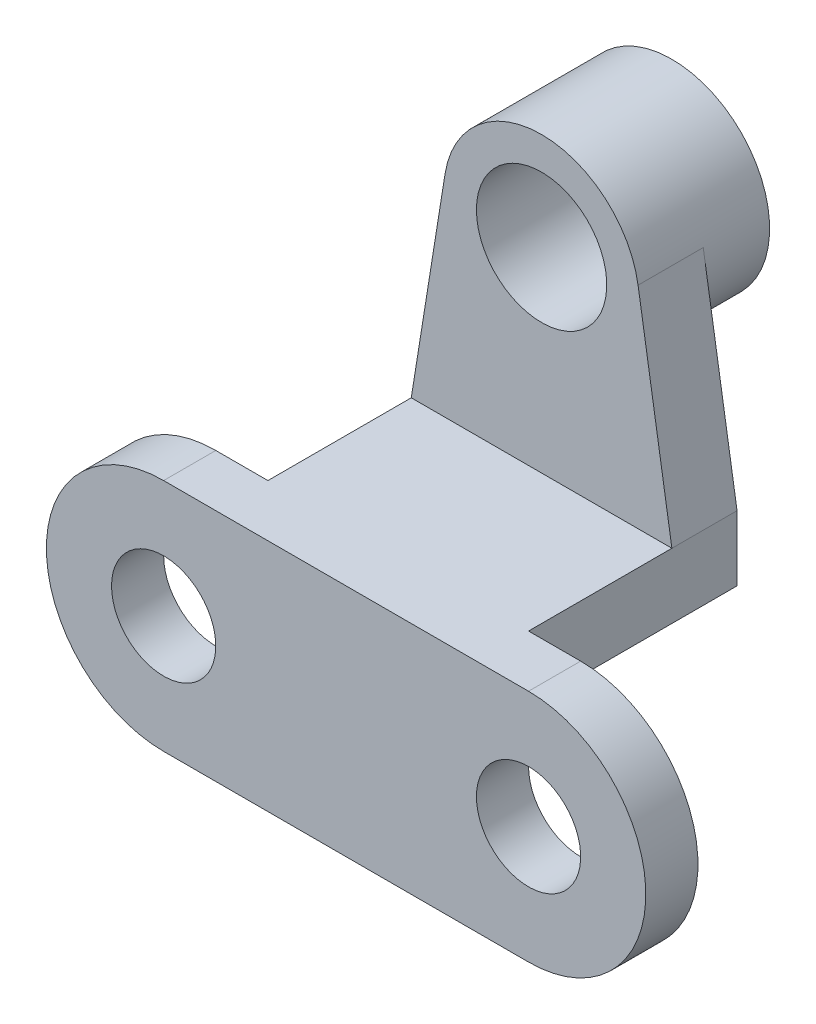
ISO-10303-21;
HEADER;
FILE_DESCRIPTION(('STEP AP214'),'2;1');
FILE_NAME('part.step','',(''),(''),'','','');
FILE_SCHEMA(('AUTOMOTIVE_DESIGN { 1 0 10303 214 1 1 1 1 }'));
ENDSEC;
DATA;
#1=APPLICATION_CONTEXT('core data for automotive mechanical design processes');
#2=APPLICATION_PROTOCOL_DEFINITION('international standard','automotive_design',2000,#1);
#3=PRODUCT_CONTEXT('',#1,'mechanical');
#4=PRODUCT('Part','Part','',(#3));
#5=PRODUCT_RELATED_PRODUCT_CATEGORY('part','',(#4));
#6=PRODUCT_DEFINITION_FORMATION('','',#4);
#7=PRODUCT_DEFINITION_CONTEXT('part definition',#1,'design');
#8=PRODUCT_DEFINITION('design','',#6,#7);
#9=PRODUCT_DEFINITION_SHAPE('','',#8);
#10=(LENGTH_UNIT() NAMED_UNIT(*) SI_UNIT(.MILLI.,.METRE.));
#11=(NAMED_UNIT(*) PLANE_ANGLE_UNIT() SI_UNIT($,.RADIAN.));
#12=(NAMED_UNIT(*) SI_UNIT($,.STERADIAN.) SOLID_ANGLE_UNIT());
#13=UNCERTAINTY_MEASURE_WITH_UNIT(LENGTH_MEASURE(1.E-05),#10,'distance_accuracy_value','');
#14=(GEOMETRIC_REPRESENTATION_CONTEXT(3) GLOBAL_UNCERTAINTY_ASSIGNED_CONTEXT((#13)) GLOBAL_UNIT_ASSIGNED_CONTEXT((#10,
#11,#12)) REPRESENTATION_CONTEXT('',''));
#15=CARTESIAN_POINT('',(0.,0.,0.));
#16=DIRECTION('',(0.,0.,1.));
#17=DIRECTION('',(1.,0.,0.));
#18=AXIS2_PLACEMENT_3D('',#15,#16,#17);
#19=CARTESIAN_POINT('',(66.,0.,0.));
#20=DIRECTION('',(0.,-0.776114000116266,-0.630592625094466));
#21=DIRECTION('',(0.,0.630592625094466,-0.776114000116266));
#22=AXIS2_PLACEMENT_3D('',#19,#20,#21);
#23=PLANE('',#22);
#24=DIRECTION('',(0.,0.630592625094466,-0.776114000116266));
#25=VECTOR('',#24,1.);
#26=CARTESIAN_POINT('',(52.,0.,0.));
#27=LINE('',#26,#25);
#28=CARTESIAN_POINT('',(52.,0.,0.));
#29=VERTEX_POINT('',#28);
#30=CARTESIAN_POINT('',(52.,26.,-32.));
#31=VERTEX_POINT('',#30);
#32=EDGE_CURVE('E199',#29,#31,#27,.T.);
#33=ORIENTED_EDGE('',*,*,#32,.F.);
#34=DIRECTION('',(-1.,0.,0.));
#35=VECTOR('',#34,1.);
#36=CARTESIAN_POINT('',(66.,0.,0.));
#37=LINE('',#36,#35);
#38=CARTESIAN_POINT('',(40.,0.,0.));
#39=VERTEX_POINT('',#38);
#40=EDGE_CURVE('E268',#29,#39,#37,.T.);
#41=ORIENTED_EDGE('',*,*,#40,.T.);
#42=DIRECTION('',(0.,-0.630592625094466,0.776114000116266));
#43=VECTOR('',#42,1.);
#44=CARTESIAN_POINT('',(40.,0.,0.));
#45=LINE('',#44,#43);
#46=CARTESIAN_POINT('',(40.,26.,-32.));
#47=VERTEX_POINT('',#46);
#48=EDGE_CURVE('E208',#47,#39,#45,.T.);
#49=ORIENTED_EDGE('',*,*,#48,.F.);
#50=DIRECTION('',(-1.,0.,0.));
#51=VECTOR('',#50,1.);
#52=CARTESIAN_POINT('',(26.,26.,-32.));
#53=LINE('',#52,#51);
#54=EDGE_CURVE('E99',#31,#47,#53,.T.);
#55=ORIENTED_EDGE('',*,*,#54,.F.);
#56=EDGE_LOOP('',(#33,#41,#49,#55));
#57=FACE_BOUND('',#56,.T.);
#58=ADVANCED_FACE('F84',(#57),#23,.T.);
#59=CARTESIAN_POINT('',(0.,0.,0.));
#60=DIRECTION('',(0.,0.,-1.));
#61=DIRECTION('',(-1.,0.,0.));
#62=AXIS2_PLACEMENT_3D('',#59,#60,#61);
#63=PLANE('',#62);
#64=DIRECTION('',(1.,0.,0.));
#65=VECTOR('',#64,1.);
#66=CARTESIAN_POINT('',(52.,26.,0.));
#67=LINE('',#66,#65);
#68=CARTESIAN_POINT('',(52.,26.,0.));
#69=VERTEX_POINT('',#68);
#70=CARTESIAN_POINT('',(66.,26.,0.));
#71=VERTEX_POINT('',#70);
#72=EDGE_CURVE('E193',#69,#71,#67,.T.);
#73=ORIENTED_EDGE('',*,*,#72,.T.);
#74=DIRECTION('',(0.,1.,0.));
#75=VECTOR('',#74,1.);
#76=CARTESIAN_POINT('',(66.,26.,0.));
#77=LINE('',#76,#75);
#78=CARTESIAN_POINT('',(66.,36.,0.));
#79=VERTEX_POINT('',#78);
#80=EDGE_CURVE('E220',#71,#79,#77,.T.);
#81=ORIENTED_EDGE('',*,*,#80,.T.);
#82=DIRECTION('',(-1.,0.,0.));
#83=VECTOR('',#82,1.);
#84=CARTESIAN_POINT('',(0.,36.,0.));
#85=LINE('',#84,#83);
#86=CARTESIAN_POINT('',(74.,36.,0.));
#87=VERTEX_POINT('',#86);
#88=EDGE_CURVE('E90',#87,#79,#85,.T.);
#89=ORIENTED_EDGE('',*,*,#88,.F.);
#90=CARTESIAN_POINT('',(74.,18.,0.));
#91=DIRECTION('',(0.,0.,1.));
#92=DIRECTION('',(1.,0.,0.));
#93=AXIS2_PLACEMENT_3D('',#90,#91,#92);
#94=CIRCLE('',#93,18.);
#95=CARTESIAN_POINT('',(74.,0.,0.));
#96=VERTEX_POINT('',#95);
#97=EDGE_CURVE('E249',#96,#87,#94,.T.);
#98=ORIENTED_EDGE('',*,*,#97,.F.);
#99=DIRECTION('',(1.,0.,0.));
#100=VECTOR('',#99,1.);
#101=CARTESIAN_POINT('',(0.,0.,0.));
#102=LINE('',#101,#100);
#103=EDGE_CURVE('E248',#29,#96,#102,.T.);
#104=ORIENTED_EDGE('',*,*,#103,.F.);
#105=DIRECTION('',(0.,-1.,0.));
#106=VECTOR('',#105,1.);
#107=CARTESIAN_POINT('',(52.,26.,0.));
#108=LINE('',#107,#106);
#109=EDGE_CURVE('E197',#69,#29,#108,.T.);
#110=ORIENTED_EDGE('',*,*,#109,.F.);
#111=EDGE_LOOP('',(#73,#81,#89,#98,#104,#110));
#112=FACE_BOUND('',#111,.T.);
#113=CARTESIAN_POINT('',(74.,18.,0.));
#114=DIRECTION('',(0.,0.,-1.));
#115=DIRECTION('',(-1.,0.,0.));
#116=AXIS2_PLACEMENT_3D('',#113,#114,#115);
#117=CIRCLE('',#116,8.);
#118=CARTESIAN_POINT('',(66.,18.,0.));
#119=VERTEX_POINT('',#118);
#120=EDGE_CURVE('E311',#119,#119,#117,.T.);
#121=ORIENTED_EDGE('',*,*,#120,.F.);
#122=EDGE_LOOP('',(#121));
#123=FACE_BOUND('',#122,.T.);
#124=ADVANCED_FACE('F275',(#112,#123),#63,.T.);
#125=CARTESIAN_POINT('',(0.,36.,8.));
#126=DIRECTION('',(0.,-1.,0.));
#127=DIRECTION('',(0.,0.,-1.));
#128=AXIS2_PLACEMENT_3D('',#125,#126,#127);
#129=PLANE('',#128);
#130=DIRECTION('',(1.,0.,0.));
#131=VECTOR('',#130,1.);
#132=CARTESIAN_POINT('',(0.,36.,-22.));
#133=LINE('',#132,#131);
#134=CARTESIAN_POINT('',(26.,36.,-22.));
#135=VERTEX_POINT('',#134);
#136=CARTESIAN_POINT('',(66.,36.,-22.));
#137=VERTEX_POINT('',#136);
#138=EDGE_CURVE('E108',#135,#137,#133,.T.);
#139=ORIENTED_EDGE('',*,*,#138,.F.);
#140=DIRECTION('',(0.,0.,1.));
#141=VECTOR('',#140,1.);
#142=CARTESIAN_POINT('',(26.,36.,0.));
#143=LINE('',#142,#141);
#144=CARTESIAN_POINT('',(26.,36.,0.));
#145=VERTEX_POINT('',#144);
#146=EDGE_CURVE('E225',#135,#145,#143,.T.);
#147=ORIENTED_EDGE('',*,*,#146,.T.);
#148=CARTESIAN_POINT('',(18.,36.,0.));
#149=VERTEX_POINT('',#148);
#150=EDGE_CURVE('E261',#145,#149,#85,.T.);
#151=ORIENTED_EDGE('',*,*,#150,.T.);
#152=DIRECTION('',(0.,0.,1.));
#153=VECTOR('',#152,1.);
#154=CARTESIAN_POINT('',(18.,36.,0.));
#155=LINE('',#154,#153);
#156=CARTESIAN_POINT('',(18.,36.,8.));
#157=VERTEX_POINT('',#156);
#158=EDGE_CURVE('E243',#149,#157,#155,.T.);
#159=ORIENTED_EDGE('',*,*,#158,.T.);
#160=DIRECTION('',(-1.,0.,0.));
#161=VECTOR('',#160,1.);
#162=CARTESIAN_POINT('',(0.,36.,8.));
#163=LINE('',#162,#161);
#164=CARTESIAN_POINT('',(74.,36.,8.));
#165=VERTEX_POINT('',#164);
#166=EDGE_CURVE('E92',#165,#157,#163,.T.);
#167=ORIENTED_EDGE('',*,*,#166,.F.);
#168=DIRECTION('',(0.,0.,1.));
#169=VECTOR('',#168,1.);
#170=CARTESIAN_POINT('',(74.,36.,0.));
#171=LINE('',#170,#169);
#172=EDGE_CURVE('E246',#87,#165,#171,.T.);
#173=ORIENTED_EDGE('',*,*,#172,.F.);
#174=ORIENTED_EDGE('',*,*,#88,.T.);
#175=DIRECTION('',(0.,0.,-1.));
#176=VECTOR('',#175,1.);
#177=CARTESIAN_POINT('',(66.,36.,-32.));
#178=LINE('',#177,#176);
#179=EDGE_CURVE('E224',#79,#137,#178,.T.);
#180=ORIENTED_EDGE('',*,*,#179,.T.);
#181=EDGE_LOOP('',(#139,#147,#151,#159,#167,#173,#174,#180));
#182=FACE_BOUND('',#181,.T.);
#183=ADVANCED_FACE('F281',(#182),#129,.F.);
#184=CARTESIAN_POINT('',(0.,0.,8.));
#185=DIRECTION('',(0.,0.,-1.));
#186=DIRECTION('',(-1.,0.,0.));
#187=AXIS2_PLACEMENT_3D('',#184,#185,#186);
#188=PLANE('',#187);
#189=CARTESIAN_POINT('',(74.,18.,8.));
#190=DIRECTION('',(0.,0.,-1.));
#191=DIRECTION('',(-1.,0.,0.));
#192=AXIS2_PLACEMENT_3D('',#189,#190,#191);
#193=CIRCLE('',#192,8.);
#194=CARTESIAN_POINT('',(66.,18.,8.));
#195=VERTEX_POINT('',#194);
#196=EDGE_CURVE('E316',#195,#195,#193,.T.);
#197=ORIENTED_EDGE('',*,*,#196,.T.);
#198=EDGE_LOOP('',(#197));
#199=FACE_BOUND('',#198,.T.);
#200=CARTESIAN_POINT('',(18.,18.,8.));
#201=DIRECTION('',(0.,0.,-1.));
#202=DIRECTION('',(-1.,0.,0.));
#203=AXIS2_PLACEMENT_3D('',#200,#201,#202);
#204=CIRCLE('',#203,8.);
#205=CARTESIAN_POINT('',(10.,18.,8.));
#206=VERTEX_POINT('',#205);
#207=EDGE_CURVE('E313',#206,#206,#204,.T.);
#208=ORIENTED_EDGE('',*,*,#207,.T.);
#209=EDGE_LOOP('',(#208));
#210=FACE_BOUND('',#209,.T.);
#211=CARTESIAN_POINT('',(18.,18.,8.));
#212=DIRECTION('',(0.,0.,1.));
#213=DIRECTION('',(1.,0.,0.));
#214=AXIS2_PLACEMENT_3D('',#211,#212,#213);
#215=CIRCLE('',#214,18.);
#216=CARTESIAN_POINT('',(18.,0.,8.));
#217=VERTEX_POINT('',#216);
#218=EDGE_CURVE('E242',#157,#217,#215,.T.);
#219=ORIENTED_EDGE('',*,*,#218,.T.);
#220=DIRECTION('',(1.,0.,0.));
#221=VECTOR('',#220,1.);
#222=CARTESIAN_POINT('',(0.,0.,8.));
#223=LINE('',#222,#221);
#224=CARTESIAN_POINT('',(74.,0.,8.));
#225=VERTEX_POINT('',#224);
#226=EDGE_CURVE('E253',#217,#225,#223,.T.);
#227=ORIENTED_EDGE('',*,*,#226,.T.);
#228=CARTESIAN_POINT('',(74.,18.,8.));
#229=DIRECTION('',(0.,0.,1.));
#230=DIRECTION('',(1.,0.,0.));
#231=AXIS2_PLACEMENT_3D('',#228,#229,#230);
#232=CIRCLE('',#231,18.);
#233=EDGE_CURVE('E238',#225,#165,#232,.T.);
#234=ORIENTED_EDGE('',*,*,#233,.T.);
#235=ORIENTED_EDGE('',*,*,#166,.T.);
#236=EDGE_LOOP('',(#219,#227,#234,#235));
#237=FACE_BOUND('',#236,.T.);
#238=ADVANCED_FACE('F278',(#199,#210,#237),#188,.F.);
#239=CARTESIAN_POINT('',(18.,18.,0.));
#240=DIRECTION('',(0.,0.,-1.));
#241=DIRECTION('',(-1.,0.,0.));
#242=AXIS2_PLACEMENT_3D('',#239,#240,#241);
#243=CIRCLE('',#242,8.);
#244=CARTESIAN_POINT('',(10.,18.,0.));
#245=VERTEX_POINT('',#244);
#246=EDGE_CURVE('E309',#245,#245,#243,.T.);
#247=ORIENTED_EDGE('',*,*,#246,.F.);
#248=EDGE_LOOP('',(#247));
#249=FACE_BOUND('',#248,.T.);
#250=DIRECTION('',(0.,1.,0.));
#251=VECTOR('',#250,1.);
#252=CARTESIAN_POINT('',(40.,26.,0.));
#253=LINE('',#252,#251);
#254=CARTESIAN_POINT('',(40.,26.,0.));
#255=VERTEX_POINT('',#254);
#256=EDGE_CURVE('E293',#39,#255,#253,.T.);
#257=ORIENTED_EDGE('',*,*,#256,.F.);
#258=CARTESIAN_POINT('',(18.,0.,0.));
#259=VERTEX_POINT('',#258);
#260=EDGE_CURVE('E256',#259,#39,#102,.T.);
#261=ORIENTED_EDGE('',*,*,#260,.F.);
#262=CARTESIAN_POINT('',(18.,18.,0.));
#263=DIRECTION('',(0.,0.,1.));
#264=DIRECTION('',(1.,0.,0.));
#265=AXIS2_PLACEMENT_3D('',#262,#263,#264);
#266=CIRCLE('',#265,18.);
#267=EDGE_CURVE('E241',#149,#259,#266,.T.);
#268=ORIENTED_EDGE('',*,*,#267,.F.);
#269=ORIENTED_EDGE('',*,*,#150,.F.);
#270=DIRECTION('',(0.,1.,0.));
#271=VECTOR('',#270,1.);
#272=CARTESIAN_POINT('',(26.,26.,0.));
#273=LINE('',#272,#271);
#274=CARTESIAN_POINT('',(26.,26.,0.));
#275=VERTEX_POINT('',#274);
#276=EDGE_CURVE('E230',#275,#145,#273,.T.);
#277=ORIENTED_EDGE('',*,*,#276,.F.);
#278=DIRECTION('',(-1.,0.,0.));
#279=VECTOR('',#278,1.);
#280=CARTESIAN_POINT('',(40.,26.,0.));
#281=LINE('',#280,#279);
#282=EDGE_CURVE('E292',#255,#275,#281,.T.);
#283=ORIENTED_EDGE('',*,*,#282,.F.);
#284=EDGE_LOOP('',(#257,#261,#268,#269,#277,#283));
#285=FACE_BOUND('',#284,.T.);
#286=ADVANCED_FACE('F289',(#249,#285),#63,.T.);
#287=CARTESIAN_POINT('',(0.,0.,8.));
#288=DIRECTION('',(0.,1.,0.));
#289=DIRECTION('',(0.,0.,1.));
#290=AXIS2_PLACEMENT_3D('',#287,#288,#289);
#291=PLANE('',#290);
#292=DIRECTION('',(0.,0.,1.));
#293=VECTOR('',#292,1.);
#294=CARTESIAN_POINT('',(18.,0.,0.));
#295=LINE('',#294,#293);
#296=EDGE_CURVE('E232',#259,#217,#295,.T.);
#297=ORIENTED_EDGE('',*,*,#296,.F.);
#298=ORIENTED_EDGE('',*,*,#260,.T.);
#299=ORIENTED_EDGE('',*,*,#40,.F.);
#300=ORIENTED_EDGE('',*,*,#103,.T.);
#301=DIRECTION('',(0.,0.,1.));
#302=VECTOR('',#301,1.);
#303=CARTESIAN_POINT('',(74.,0.,0.));
#304=LINE('',#303,#302);
#305=EDGE_CURVE('E233',#96,#225,#304,.T.);
#306=ORIENTED_EDGE('',*,*,#305,.T.);
#307=ORIENTED_EDGE('',*,*,#226,.F.);
#308=EDGE_LOOP('',(#297,#298,#299,#300,#306,#307));
#309=FACE_BOUND('',#308,.T.);
#310=ADVANCED_FACE('F83',(#309),#291,.F.);
#311=CARTESIAN_POINT('',(74.,18.,0.));
#312=DIRECTION('',(0.,0.,1.));
#313=DIRECTION('',(1.,0.,0.));
#314=AXIS2_PLACEMENT_3D('',#311,#312,#313);
#315=CYLINDRICAL_SURFACE('',#314,18.);
#316=ORIENTED_EDGE('',*,*,#233,.F.);
#317=ORIENTED_EDGE('',*,*,#305,.F.);
#318=ORIENTED_EDGE('',*,*,#97,.T.);
#319=ORIENTED_EDGE('',*,*,#172,.T.);
#320=EDGE_LOOP('',(#316,#317,#318,#319));
#321=FACE_BOUND('',#320,.T.);
#322=ADVANCED_FACE('F280',(#321),#315,.T.);
#323=CARTESIAN_POINT('',(18.,18.,0.));
#324=DIRECTION('',(0.,0.,1.));
#325=DIRECTION('',(1.,0.,0.));
#326=AXIS2_PLACEMENT_3D('',#323,#324,#325);
#327=CYLINDRICAL_SURFACE('',#326,18.);
#328=ORIENTED_EDGE('',*,*,#218,.F.);
#329=ORIENTED_EDGE('',*,*,#158,.F.);
#330=ORIENTED_EDGE('',*,*,#267,.T.);
#331=ORIENTED_EDGE('',*,*,#296,.T.);
#332=EDGE_LOOP('',(#328,#329,#330,#331));
#333=FACE_BOUND('',#332,.T.);
#334=ADVANCED_FACE('F286',(#333),#327,.T.);
#335=CARTESIAN_POINT('',(26.,26.,0.));
#336=DIRECTION('',(-1.,0.,0.));
#337=DIRECTION('',(0.,0.,1.));
#338=AXIS2_PLACEMENT_3D('',#335,#336,#337);
#339=PLANE('',#338);
#340=DIRECTION('',(0.,0.,-1.));
#341=VECTOR('',#340,1.);
#342=CARTESIAN_POINT('',(26.,26.,-32.));
#343=LINE('',#342,#341);
#344=CARTESIAN_POINT('',(26.,26.,-32.));
#345=VERTEX_POINT('',#344);
#346=EDGE_CURVE('E299',#275,#345,#343,.T.);
#347=ORIENTED_EDGE('',*,*,#346,.F.);
#348=ORIENTED_EDGE('',*,*,#276,.T.);
#349=ORIENTED_EDGE('',*,*,#146,.F.);
#350=CARTESIAN_POINT('',(26.,36.,-32.));
#351=VERTEX_POINT('',#350);
#352=EDGE_CURVE('E212',#351,#135,#143,.T.);
#353=ORIENTED_EDGE('',*,*,#352,.F.);
#354=DIRECTION('',(0.,1.,0.));
#355=VECTOR('',#354,1.);
#356=CARTESIAN_POINT('',(26.,26.,-32.));
#357=LINE('',#356,#355);
#358=EDGE_CURVE('E235',#345,#351,#357,.T.);
#359=ORIENTED_EDGE('',*,*,#358,.F.);
#360=EDGE_LOOP('',(#347,#348,#349,#353,#359));
#361=FACE_BOUND('',#360,.T.);
#362=ADVANCED_FACE('F417',(#361),#339,.T.);
#363=CARTESIAN_POINT('',(26.,26.,-32.));
#364=DIRECTION('',(0.,0.,-1.));
#365=DIRECTION('',(-1.,0.,0.));
#366=AXIS2_PLACEMENT_3D('',#363,#364,#365);
#367=PLANE('',#366);
#368=CARTESIAN_POINT('',(46.,66.,-32.));
#369=DIRECTION('',(0.,0.,-1.));
#370=DIRECTION('',(-1.,0.,0.));
#371=AXIS2_PLACEMENT_3D('',#368,#369,#370);
#372=CIRCLE('',#371,15.);
#373=CARTESIAN_POINT('',(60.8109512920612,68.3739675280408,-32.));
#374=VERTEX_POINT('',#373);
#375=CARTESIAN_POINT('',(31.1890487079389,68.3739675280408,-32.));
#376=VERTEX_POINT('',#375);
#377=EDGE_CURVE('E12',#374,#376,#372,.T.);
#378=ORIENTED_EDGE('',*,*,#377,.F.);
#379=DIRECTION('',(-0.158264501869386,0.987396752804077,0.));
#380=VECTOR('',#379,1.);
#381=CARTESIAN_POINT('',(69.9725697198499,11.2155259370498,-32.));
#382=LINE('',#381,#380);
#383=CARTESIAN_POINT('',(66.,36.,-32.));
#384=VERTEX_POINT('',#383);
#385=EDGE_CURVE('E329',#384,#374,#382,.T.);
#386=ORIENTED_EDGE('',*,*,#385,.F.);
#387=DIRECTION('',(0.,1.,0.));
#388=VECTOR('',#387,1.);
#389=CARTESIAN_POINT('',(66.,26.,-32.));
#390=LINE('',#389,#388);
#391=CARTESIAN_POINT('',(66.,26.,-32.));
#392=VERTEX_POINT('',#391);
#393=EDGE_CURVE('E216',#392,#384,#390,.T.);
#394=ORIENTED_EDGE('',*,*,#393,.F.);
#395=EDGE_CURVE('E194',#392,#31,#53,.T.);
#396=ORIENTED_EDGE('',*,*,#395,.T.);
#397=ORIENTED_EDGE('',*,*,#54,.T.);
#398=DIRECTION('',(-1.,0.,0.));
#399=VECTOR('',#398,1.);
#400=CARTESIAN_POINT('',(40.,26.,-32.));
#401=LINE('',#400,#399);
#402=EDGE_CURVE('E306',#47,#345,#401,.T.);
#403=ORIENTED_EDGE('',*,*,#402,.T.);
#404=ORIENTED_EDGE('',*,*,#358,.T.);
#405=DIRECTION('',(0.158264501869385,0.987396752804077,0.));
#406=VECTOR('',#405,1.);
#407=CARTESIAN_POINT('',(19.7230462453695,-3.1613007441089,-32.));
#408=LINE('',#407,#406);
#409=EDGE_CURVE('E337',#351,#376,#408,.T.);
#410=ORIENTED_EDGE('',*,*,#409,.T.);
#411=EDGE_LOOP('',(#378,#386,#394,#396,#397,#403,#404,#410));
#412=FACE_BOUND('',#411,.T.);
#413=ADVANCED_FACE('F211',(#412),#367,.T.);
#414=CARTESIAN_POINT('',(66.,26.,-32.));
#415=DIRECTION('',(1.,0.,0.));
#416=DIRECTION('',(0.,0.,-1.));
#417=AXIS2_PLACEMENT_3D('',#414,#415,#416);
#418=PLANE('',#417);
#419=DIRECTION('',(0.,0.,1.));
#420=VECTOR('',#419,1.);
#421=CARTESIAN_POINT('',(66.,26.,-32.));
#422=LINE('',#421,#420);
#423=EDGE_CURVE('E207',#392,#71,#422,.T.);
#424=ORIENTED_EDGE('',*,*,#423,.F.);
#425=ORIENTED_EDGE('',*,*,#393,.T.);
#426=DIRECTION('',(0.,0.,-1.));
#427=VECTOR('',#426,1.);
#428=CARTESIAN_POINT('',(66.,36.,-22.));
#429=LINE('',#428,#427);
#430=EDGE_CURVE('E346',#137,#384,#429,.T.);
#431=ORIENTED_EDGE('',*,*,#430,.F.);
#432=ORIENTED_EDGE('',*,*,#179,.F.);
#433=ORIENTED_EDGE('',*,*,#80,.F.);
#434=EDGE_LOOP('',(#424,#425,#431,#432,#433));
#435=FACE_BOUND('',#434,.T.);
#436=ADVANCED_FACE('F409',(#435),#418,.T.);
#437=CARTESIAN_POINT('',(46.,66.,-22.));
#438=DIRECTION('',(0.,0.,-1.));
#439=DIRECTION('',(-1.,0.,0.));
#440=AXIS2_PLACEMENT_3D('',#437,#438,#439);
#441=CYLINDRICAL_SURFACE('',#440,15.);
#442=DIRECTION('',(0.,0.,-1.));
#443=VECTOR('',#442,1.);
#444=CARTESIAN_POINT('',(60.8109512920612,68.3739675280408,-22.));
#445=LINE('',#444,#443);
#446=CARTESIAN_POINT('',(60.8109512920612,68.3739675280408,-22.));
#447=VERTEX_POINT('',#446);
#448=EDGE_CURVE('E221',#447,#374,#445,.T.);
#449=ORIENTED_EDGE('',*,*,#448,.T.);
#450=ORIENTED_EDGE('',*,*,#377,.T.);
#451=DIRECTION('',(0.,0.,-1.));
#452=VECTOR('',#451,1.);
#453=CARTESIAN_POINT('',(31.1890487079389,68.3739675280408,-22.));
#454=LINE('',#453,#452);
#455=CARTESIAN_POINT('',(31.1890487079389,68.3739675280408,-22.));
#456=VERTEX_POINT('',#455);
#457=EDGE_CURVE('E228',#456,#376,#454,.T.);
#458=ORIENTED_EDGE('',*,*,#457,.F.);
#459=CARTESIAN_POINT('',(46.,66.,-22.));
#460=DIRECTION('',(0.,0.,-1.));
#461=DIRECTION('',(-1.,0.,0.));
#462=AXIS2_PLACEMENT_3D('',#459,#460,#461);
#463=CIRCLE('',#462,15.);
#464=EDGE_CURVE('E332',#456,#447,#463,.T.);
#465=ORIENTED_EDGE('',*,*,#464,.T.);
#466=EDGE_LOOP('',(#449,#450,#458,#465));
#467=FACE_BOUND('',#466,.T.);
#468=CARTESIAN_POINT('',(46.,66.,-42.));
#469=DIRECTION('',(0.,0.,-1.));
#470=DIRECTION('',(-1.,0.,0.));
#471=AXIS2_PLACEMENT_3D('',#468,#469,#470);
#472=CIRCLE('',#471,15.);
#473=CARTESIAN_POINT('',(31.,66.,-42.));
#474=VERTEX_POINT('',#473);
#475=EDGE_CURVE('E326',#474,#474,#472,.T.);
#476=ORIENTED_EDGE('',*,*,#475,.F.);
#477=EDGE_LOOP('',(#476));
#478=FACE_BOUND('',#477,.T.);
#479=ADVANCED_FACE('F354',(#467,#478),#441,.T.);
#480=CARTESIAN_POINT('',(19.7230462453695,-3.1613007441089,-22.));
#481=DIRECTION('',(-0.987396752804077,0.158264501869385,0.));
#482=DIRECTION('',(-0.158264501869385,-0.987396752804077,0.));
#483=AXIS2_PLACEMENT_3D('',#480,#481,#482);
#484=PLANE('',#483);
#485=ORIENTED_EDGE('',*,*,#409,.F.);
#486=ORIENTED_EDGE('',*,*,#352,.T.);
#487=DIRECTION('',(0.158264501869385,0.987396752804077,0.));
#488=VECTOR('',#487,1.);
#489=CARTESIAN_POINT('',(19.7230462453695,-3.1613007441089,-22.));
#490=LINE('',#489,#488);
#491=EDGE_CURVE('E339',#135,#456,#490,.T.);
#492=ORIENTED_EDGE('',*,*,#491,.T.);
#493=ORIENTED_EDGE('',*,*,#457,.T.);
#494=EDGE_LOOP('',(#485,#486,#492,#493));
#495=FACE_BOUND('',#494,.T.);
#496=ADVANCED_FACE('F363',(#495),#484,.T.);
#497=CARTESIAN_POINT('',(69.9725697198499,11.2155259370498,-22.));
#498=DIRECTION('',(-0.987396752804077,-0.158264501869386,0.));
#499=DIRECTION('',(0.158264501869386,-0.987396752804077,0.));
#500=AXIS2_PLACEMENT_3D('',#497,#498,#499);
#501=PLANE('',#500);
#502=ORIENTED_EDGE('',*,*,#385,.T.);
#503=ORIENTED_EDGE('',*,*,#448,.F.);
#504=DIRECTION('',(-0.158264501869386,0.987396752804077,0.));
#505=VECTOR('',#504,1.);
#506=CARTESIAN_POINT('',(69.9725697198499,11.2155259370498,-22.));
#507=LINE('',#506,#505);
#508=EDGE_CURVE('E335',#137,#447,#507,.T.);
#509=ORIENTED_EDGE('',*,*,#508,.F.);
#510=ORIENTED_EDGE('',*,*,#430,.T.);
#511=EDGE_LOOP('',(#502,#503,#509,#510));
#512=FACE_BOUND('',#511,.T.);
#513=ADVANCED_FACE('F358',(#512),#501,.F.);
#514=CARTESIAN_POINT('',(0.,0.,-22.));
#515=DIRECTION('',(0.,0.,-1.));
#516=DIRECTION('',(-1.,0.,0.));
#517=AXIS2_PLACEMENT_3D('',#514,#515,#516);
#518=PLANE('',#517);
#519=CARTESIAN_POINT('',(46.,66.,-22.));
#520=DIRECTION('',(0.,0.,-1.));
#521=DIRECTION('',(-1.,0.,0.));
#522=AXIS2_PLACEMENT_3D('',#519,#520,#521);
#523=CIRCLE('',#522,10.);
#524=CARTESIAN_POINT('',(36.,66.,-22.));
#525=VERTEX_POINT('',#524);
#526=EDGE_CURVE('E324',#525,#525,#523,.T.);
#527=ORIENTED_EDGE('',*,*,#526,.T.);
#528=EDGE_LOOP('',(#527));
#529=FACE_BOUND('',#528,.T.);
#530=ORIENTED_EDGE('',*,*,#464,.F.);
#531=ORIENTED_EDGE('',*,*,#491,.F.);
#532=ORIENTED_EDGE('',*,*,#138,.T.);
#533=ORIENTED_EDGE('',*,*,#508,.T.);
#534=EDGE_LOOP('',(#530,#531,#532,#533));
#535=FACE_BOUND('',#534,.T.);
#536=ADVANCED_FACE('F364',(#529,#535),#518,.F.);
#537=CARTESIAN_POINT('',(46.,66.,-42.));
#538=DIRECTION('',(0.,0.,-1.));
#539=DIRECTION('',(-1.,0.,0.));
#540=AXIS2_PLACEMENT_3D('',#537,#538,#539);
#541=PLANE('',#540);
#542=CARTESIAN_POINT('',(46.,66.,-42.));
#543=DIRECTION('',(0.,0.,-1.));
#544=DIRECTION('',(-1.,0.,0.));
#545=AXIS2_PLACEMENT_3D('',#542,#543,#544);
#546=CIRCLE('',#545,10.);
#547=CARTESIAN_POINT('',(36.,66.,-42.));
#548=VERTEX_POINT('',#547);
#549=EDGE_CURVE('E325',#548,#548,#546,.T.);
#550=ORIENTED_EDGE('',*,*,#549,.F.);
#551=EDGE_LOOP('',(#550));
#552=FACE_BOUND('',#551,.T.);
#553=ORIENTED_EDGE('',*,*,#475,.T.);
#554=EDGE_LOOP('',(#553));
#555=FACE_BOUND('',#554,.T.);
#556=ADVANCED_FACE('F366',(#552,#555),#541,.T.);
#557=CARTESIAN_POINT('',(46.,66.,-22.));
#558=DIRECTION('',(0.,0.,-1.));
#559=DIRECTION('',(-1.,0.,0.));
#560=AXIS2_PLACEMENT_3D('',#557,#558,#559);
#561=CYLINDRICAL_SURFACE('',#560,10.);
#562=ORIENTED_EDGE('',*,*,#526,.F.);
#563=EDGE_LOOP('',(#562));
#564=FACE_BOUND('',#563,.T.);
#565=ORIENTED_EDGE('',*,*,#549,.T.);
#566=EDGE_LOOP('',(#565));
#567=FACE_BOUND('',#566,.T.);
#568=ADVANCED_FACE('F372',(#564,#567),#561,.F.);
#569=CARTESIAN_POINT('',(18.,18.,20.));
#570=DIRECTION('',(0.,0.,-1.));
#571=DIRECTION('',(-1.,0.,0.));
#572=AXIS2_PLACEMENT_3D('',#569,#570,#571);
#573=CYLINDRICAL_SURFACE('',#572,8.);
#574=ORIENTED_EDGE('',*,*,#246,.T.);
#575=EDGE_LOOP('',(#574));
#576=FACE_BOUND('',#575,.T.);
#577=ORIENTED_EDGE('',*,*,#207,.F.);
#578=EDGE_LOOP('',(#577));
#579=FACE_BOUND('',#578,.T.);
#580=ADVANCED_FACE('F393',(#576,#579),#573,.F.);
#581=CARTESIAN_POINT('',(74.,18.,20.));
#582=DIRECTION('',(0.,0.,-1.));
#583=DIRECTION('',(-1.,0.,0.));
#584=AXIS2_PLACEMENT_3D('',#581,#582,#583);
#585=CYLINDRICAL_SURFACE('',#584,8.);
#586=ORIENTED_EDGE('',*,*,#120,.T.);
#587=EDGE_LOOP('',(#586));
#588=FACE_BOUND('',#587,.T.);
#589=ORIENTED_EDGE('',*,*,#196,.F.);
#590=EDGE_LOOP('',(#589));
#591=FACE_BOUND('',#590,.T.);
#592=ADVANCED_FACE('F388',(#588,#591),#585,.F.);
#593=CARTESIAN_POINT('',(40.,26.,-32.));
#594=DIRECTION('',(0.,1.,0.));
#595=DIRECTION('',(0.,0.,1.));
#596=AXIS2_PLACEMENT_3D('',#593,#594,#595);
#597=PLANE('',#596);
#598=ORIENTED_EDGE('',*,*,#346,.T.);
#599=ORIENTED_EDGE('',*,*,#402,.F.);
#600=DIRECTION('',(0.,0.,-1.));
#601=VECTOR('',#600,1.);
#602=CARTESIAN_POINT('',(40.,26.,-32.));
#603=LINE('',#602,#601);
#604=EDGE_CURVE('E294',#255,#47,#603,.T.);
#605=ORIENTED_EDGE('',*,*,#604,.F.);
#606=ORIENTED_EDGE('',*,*,#282,.T.);
#607=EDGE_LOOP('',(#598,#599,#605,#606));
#608=FACE_BOUND('',#607,.T.);
#609=ADVANCED_FACE('F389',(#608),#597,.F.);
#610=CARTESIAN_POINT('',(40.,0.,0.));
#611=DIRECTION('',(-1.,0.,0.));
#612=DIRECTION('',(0.,0.,1.));
#613=AXIS2_PLACEMENT_3D('',#610,#611,#612);
#614=PLANE('',#613);
#615=ORIENTED_EDGE('',*,*,#48,.T.);
#616=ORIENTED_EDGE('',*,*,#256,.T.);
#617=ORIENTED_EDGE('',*,*,#604,.T.);
#618=EDGE_LOOP('',(#615,#616,#617));
#619=FACE_BOUND('',#618,.T.);
#620=ADVANCED_FACE('F300',(#619),#614,.T.);
#621=CARTESIAN_POINT('',(52.,26.,-32.));
#622=DIRECTION('',(0.,1.,0.));
#623=DIRECTION('',(0.,0.,1.));
#624=AXIS2_PLACEMENT_3D('',#621,#622,#623);
#625=PLANE('',#624);
#626=ORIENTED_EDGE('',*,*,#423,.T.);
#627=ORIENTED_EDGE('',*,*,#72,.F.);
#628=DIRECTION('',(0.,0.,1.));
#629=VECTOR('',#628,1.);
#630=CARTESIAN_POINT('',(52.,26.,-32.));
#631=LINE('',#630,#629);
#632=EDGE_CURVE('E186',#31,#69,#631,.T.);
#633=ORIENTED_EDGE('',*,*,#632,.F.);
#634=ORIENTED_EDGE('',*,*,#395,.F.);
#635=EDGE_LOOP('',(#626,#627,#633,#634));
#636=FACE_BOUND('',#635,.T.);
#637=ADVANCED_FACE('F195',(#636),#625,.F.);
#638=CARTESIAN_POINT('',(52.,0.,0.));
#639=DIRECTION('',(-1.,0.,0.));
#640=DIRECTION('',(0.,0.,1.));
#641=AXIS2_PLACEMENT_3D('',#638,#639,#640);
#642=PLANE('',#641);
#643=ORIENTED_EDGE('',*,*,#32,.T.);
#644=ORIENTED_EDGE('',*,*,#632,.T.);
#645=ORIENTED_EDGE('',*,*,#109,.T.);
#646=EDGE_LOOP('',(#643,#644,#645));
#647=FACE_BOUND('',#646,.T.);
#648=ADVANCED_FACE('F204',(#647),#642,.F.);
#649=CLOSED_SHELL('',(#58,#124,#183,#238,#286,#310,#322,#334,#362,#413,#436,#479,#496,#513,#536,
#556,#568,#580,#592,#609,#620,#637,#648));
#650=MANIFOLD_SOLID_BREP('B2',#649);
#651=ADVANCED_BREP_SHAPE_REPRESENTATION('',(#18,#650),#14);
#652=SHAPE_DEFINITION_REPRESENTATION(#9,#651);
ENDSEC;
END-ISO-10303-21;
